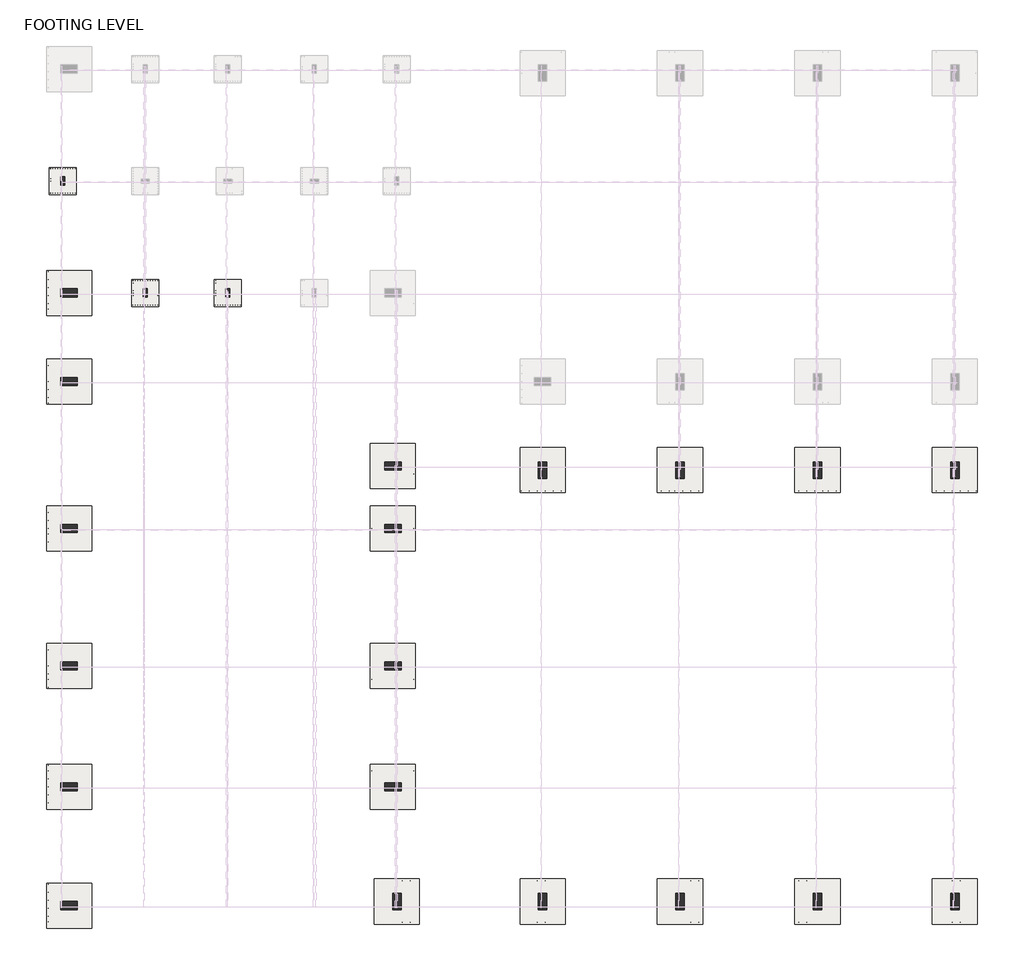
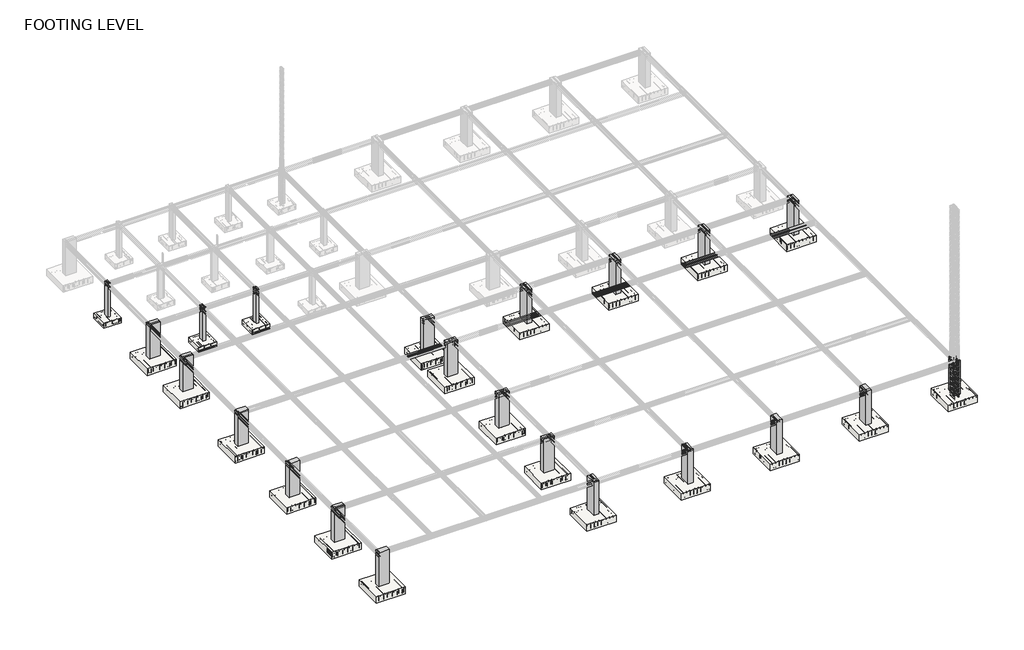
# One storey, part 1 of 19: 22 columns, 22 slabs.
"""IFC4 building model written with IfcOpenShell, lengths in millimetres."""

from ifc_helpers import new_model, si_unit, frame, origin, place, context, project, spatial, polyline, outline, extrude, faceted_brep, transform, mapped, element, save
from components import m_footing_rectangular_2500_x_2500_x_600_5d9c2050

model = new_model("IFC4")

# Units and contexts
model_context = context("Model", 3, world=origin())
ifc_project = project(units=[si_unit("LENGTHUNIT", "METRE", prefix="MILLI")], contexts=[model_context])

# Site, building, storey
site = spatial("IfcSite", under=ifc_project)
building = spatial("IfcBuilding", under=site)
storey = spatial("IfcBuildingStorey", under=building, Name="FOOTING LEVEL", Elevation=-3048.0)

# Columns
placement = place(None, origin())
element("IfcColumn", 1, ObjectType="M_Concrete-Rectangular-Column : 18\" X 36\"", at=placement, inside=storey, context=model_context, shape_type="SweptSolid", body=[
    extrude(outline(polyline([(32541.1587563, -27373.8205555), (32541.1587563, -28288.2205555), (32083.9587563, -28288.2205555), (32083.9587563, -27373.8205555), (32541.1587563, -27373.8205555)])), frame((0.0, 0.0, -3048.0), z_axis=(0.0, 0.0, 1.0), x_axis=(1.0, 0.0, 0.0)), (0.0, 0.0, 1.0), 3048.0),
])
element("IfcColumn", 2, ObjectType="M_Concrete-Rectangular-Column : 18\" X 36\"", at=placement, inside=storey, context=model_context, shape_type="SweptSolid", body=[
    extrude(outline(polyline([(24921.1587563, -27373.8205555), (24921.1587563, -28288.2205555), (24463.9587563, -28288.2205555), (24463.9587563, -27373.8205555), (24921.1587563, -27373.8205555)])), frame((0.0, 0.0, -3048.0), z_axis=(0.0, 0.0, 1.0), x_axis=(1.0, 0.0, 0.0)), (0.0, 0.0, 1.0), 3048.0),
])
element("IfcColumn", 3, ObjectType="M_Concrete-Rectangular-Column : 18\" X 36\"", at=placement, inside=storey, context=model_context, shape_type="Brep", body=[
    faceted_brep([(17301.1587563, -27373.8205555, -3048.0), (17301.1587563, -28288.2205555, -3048.0), (16843.9587563, -28288.2205555, -3048.0), (16843.9587563, -27373.8205555, -3048.0), (17301.1587563, -27373.8205555, 0.0), (17301.1587563, -27945.3205555, 0.0), (17301.1587563, -28173.9205555, 0.0), (17301.1587563, -28288.2205555, 0.0), (16843.9587563, -28288.2205555, 0.0), (16843.9587563, -28173.9205555, 0.0), (16843.9587563, -27945.3205555, 0.0), (16843.9587563, -27373.8205555, 0.0)], [[[0, 1, 2, 3]], [[4, 5, 6, 7, 1, 0]], [[7, 8, 2, 1]], [[8, 9, 10, 11, 3, 2]], [[11, 4, 0, 3]], [[4, 11, 10, 9, 8, 7, 6, 5]]]),
])
element("IfcColumn", 4, ObjectType="M_Concrete-Rectangular-Column : 18\" X 36\"", at=placement, inside=storey, context=model_context, shape_type="Brep", body=[
    faceted_brep([(9681.1587563, -27373.8205555, -3048.0), (9681.1587563, -28288.2205555, -3048.0), (9223.9587563, -28288.2205555, -3048.0), (9223.9587563, -27373.8205555, -3048.0), (9681.1587563, -27373.8205555, 0.0), (9681.1587563, -27945.3205555, 0.0), (9681.1587563, -28173.9205555, 0.0), (9681.1587563, -28288.2205555, 0.0), (9223.9587563, -28288.2205555, 0.0), (9223.9587563, -28173.9205555, 0.0), (9223.9587563, -27945.3205555, 0.0), (9223.9587563, -27373.8205555, 0.0)], [[[0, 1, 2, 3]], [[4, 5, 6, 7, 1, 0]], [[7, 8, 2, 1]], [[8, 9, 10, 11, 3, 2]], [[11, 4, 0, 3]], [[4, 11, 10, 9, 8, 7, 6, 5]]]),
])
element("IfcColumn", 5, ObjectType="M_Concrete-Rectangular-Column : 18\" X 36\"", at=placement, inside=storey, context=model_context, shape_type="SweptSolid", body=[
    extrude(outline(polyline([(1603.9587563, -27373.8205555), (1603.9587563, -28288.2205555), (1146.7587563, -28288.2205555), (1146.7587563, -27373.8205555), (1603.9587563, -27373.8205555)])), frame((0.0, 0.0, -3048.0), z_axis=(0.0, 0.0, 1.0), x_axis=(1.0, 0.0, 0.0)), (0.0, 0.0, 1.0), 3048.0),
])
element("IfcColumn", 6, ObjectType="M_Concrete-Rectangular-Column : 18\" X 36\"", at=placement, inside=storey, context=model_context, shape_type="SweptSolid", body=[
    extrude(outline(polyline([(-17255.5412437, -27831.0205555), (-16341.1412437, -27831.0205555), (-16341.1412437, -28288.2205555), (-17255.5412437, -28288.2205555), (-17255.5412437, -27831.0205555)])), frame((0.0, 0.0, -3048.0), z_axis=(0.0, 0.0, 1.0), x_axis=(1.0, 0.0, 0.0)), (0.0, 0.0, 1.0), 3048.0),
])
element("IfcColumn", 7, ObjectType="M_Concrete-Rectangular-Column : 18\" X 36\"", at=placement, inside=storey, context=model_context, shape_type="Brep", body=[
    faceted_brep([(-17255.5412437, -21239.7205555, -3048.0), (-16341.1412437, -21239.7205555, -3048.0), (-16341.1412437, -21696.9205555, -3048.0), (-17255.5412437, -21696.9205555, -3048.0), (-17255.5412437, -21239.7205555, 0.0), (-17026.9412437, -21239.7205555, 0.0), (-16341.1412437, -21239.7205555, 0.0), (-17255.5412437, -21239.7205555, -457.2), (-16341.1412437, -21696.9205555, 0.0), (-17026.9412437, -21696.9205555, 0.0), (-17255.5412437, -21696.9205555, 0.0), (-17255.5412437, -21696.9205555, -457.2)], [[[0, 1, 2, 3]], [[4, 5, 6, 1, 0, 7]], [[6, 8, 2, 1]], [[8, 9, 10, 11, 3, 2]], [[10, 4, 7, 0, 3, 11]], [[4, 10, 9, 8, 6, 5]]]),
])
element("IfcColumn", 8, ObjectType="M_Concrete-Rectangular-Column : 18\" X 36\"", at=placement, inside=storey, context=model_context, shape_type="Brep", body=[
    faceted_brep([(-17255.5412437, -14534.1205555, -3048.0), (-16341.1412437, -14534.1205555, -3048.0), (-16341.1412437, -14991.3205555, -3048.0), (-17255.5412437, -14991.3205555, -3048.0), (-17255.5412437, -14534.1205555, 0.0), (-17026.9412437, -14534.1205555, 0.0), (-16341.1412437, -14534.1205555, 0.0), (-17255.5412437, -14534.1205555, -457.2), (-16341.1412437, -14991.3205555, 0.0), (-17026.9412437, -14991.3205555, 0.0), (-17255.5412437, -14991.3205555, 0.0), (-17255.5412437, -14991.3205555, -457.2)], [[[0, 1, 2, 3]], [[4, 5, 6, 1, 0, 7]], [[6, 8, 2, 1]], [[8, 9, 10, 11, 3, 2]], [[10, 4, 7, 0, 3, 11]], [[4, 10, 9, 8, 6, 5]]]),
])
element("IfcColumn", 9, ObjectType="M_Concrete-Rectangular-Column : 18\" X 36\"", at=placement, inside=storey, context=model_context, shape_type="Brep", body=[
    faceted_brep([(-17255.5412437, -6914.1205555, -3048.0), (-16341.1412437, -6914.1205555, -3048.0), (-16341.1412437, -7371.3205555, -3048.0), (-17255.5412437, -7371.3205555, -3048.0), (-17255.5412437, -6914.1205555, 0.0), (-17026.9412437, -6914.1205555, 0.0), (-16341.1412437, -6914.1205555, 0.0), (-17255.5412437, -6914.1205555, -457.2), (-16341.1412437, -7371.3205555, 0.0), (-17026.9412437, -7371.3205555, 0.0), (-17255.5412437, -7371.3205555, 0.0), (-17255.5412437, -7371.3205555, -457.2)], [[[0, 1, 2, 3]], [[4, 5, 6, 1, 0, 7]], [[6, 8, 2, 1]], [[8, 9, 10, 11, 3, 2]], [[10, 4, 7, 0, 3, 11]], [[4, 10, 9, 8, 6, 5]]]),
])
element("IfcColumn", 10, ObjectType="M_Concrete-Rectangular-Column : 18\" X 36\"", at=placement, inside=storey, context=model_context, shape_type="Brep", body=[
    faceted_brep([(-17255.5412437, 1239.2794445, -3048.0), (-16341.1412437, 1239.2794445, -3048.0), (-16341.1412437, 782.0794445, -3048.0), (-17255.5412437, 782.0794445, -3048.0), (-17255.5412437, 1239.2794445, 0.0), (-17026.9412437, 1239.2794445, 0.0), (-16341.1412437, 1239.2794445, 0.0), (-17255.5412437, 1239.2794445, -457.2), (-16341.1412437, 782.0794445, 0.0), (-17026.9412437, 782.0794445, 0.0), (-17255.5412437, 782.0794445, 0.0), (-17255.5412437, 782.0794445, -457.2)], [[[0, 1, 2, 3]], [[4, 5, 6, 1, 0, 7]], [[6, 8, 2, 1]], [[8, 9, 10, 11, 3, 2]], [[10, 4, 7, 0, 3, 11]], [[4, 10, 9, 8, 6, 5]]]),
])
element("IfcColumn", 11, ObjectType="M_Concrete-Rectangular-Column : 18\" X 36\"", at=placement, inside=storey, context=model_context, shape_type="SweptSolid", body=[
    extrude(outline(polyline([(-17255.5412437, 6154.1794445), (-16341.1412437, 6154.1794445), (-16341.1412437, 5696.9794445), (-17255.5412437, 5696.9794445), (-17255.5412437, 6154.1794445)])), frame((0.0, 0.0, -3048.0), z_axis=(0.0, 0.0, 1.0), x_axis=(1.0, 0.0, 0.0)), (0.0, 0.0, 1.0), 3048.0),
])
element("IfcColumn", 12, ObjectType="M_Concrete-Rectangular-Column : 18\" X 36\"", at=placement, inside=storey, context=model_context, shape_type="Brep", body=[
    faceted_brep([(689.5587563, -3447.0205555, -3048.0), (1603.9587563, -3447.0205555, -3048.0), (1603.9587563, -3904.2205555, -3048.0), (689.5587563, -3904.2205555, -3048.0), (689.5587563, -3447.0205555, 0.0), (1261.0587563, -3447.0205555, 0.0), (1489.6587563, -3447.0205555, 0.0), (1603.9587563, -3447.0205555, 0.0), (1603.9587563, -3904.2205555, 0.0), (1489.6587563, -3904.2205555, 0.0), (1261.0587563, -3904.2205555, 0.0), (689.5587563, -3904.2205555, 0.0)], [[[0, 1, 2, 3]], [[4, 5, 6, 7, 1, 0]], [[7, 8, 2, 1]], [[8, 9, 10, 11, 3, 2]], [[11, 4, 0, 3]], [[4, 11, 10, 9, 8, 7, 6, 5]]]),
])
element("IfcColumn", 13, ObjectType="M_Concrete-Rectangular-Column : 18\" X 36\"", at=placement, inside=storey, context=model_context, shape_type="SweptSolid", body=[
    extrude(outline(polyline([(689.5587563, -6914.1205555), (1603.9587563, -6914.1205555), (1603.9587563, -7371.3205555), (689.5587563, -7371.3205555), (689.5587563, -6914.1205555)])), frame((0.0, 0.0, -3048.0), z_axis=(0.0, 0.0, 1.0), x_axis=(1.0, 0.0, 0.0)), (0.0, 0.0, 1.0), 3048.0),
])
element("IfcColumn", 14, ObjectType="M_Concrete-Rectangular-Column : 18\" X 36\"", at=placement, inside=storey, context=model_context, shape_type="Brep", body=[
    faceted_brep([(689.5587563, -14534.1205555, -3048.0), (1603.9587563, -14534.1205555, -3048.0), (1603.9587563, -14991.3205555, -3048.0), (689.5587563, -14991.3205555, -3048.0), (689.5587563, -14534.1205555, 0.0), (1261.0587563, -14534.1205555, 0.0), (1489.6587563, -14534.1205555, 0.0), (1603.9587563, -14534.1205555, 0.0), (1603.9587563, -14991.3205555, 0.0), (1489.6587563, -14991.3205555, 0.0), (1261.0587563, -14991.3205555, 0.0), (689.5587563, -14991.3205555, 0.0)], [[[0, 1, 2, 3]], [[4, 5, 6, 7, 1, 0]], [[7, 8, 2, 1]], [[8, 9, 10, 11, 3, 2]], [[11, 4, 0, 3]], [[4, 11, 10, 9, 8, 7, 6, 5]]]),
])
element("IfcColumn", 15, ObjectType="M_Concrete-Rectangular-Column : 18\" X 36\"", at=placement, inside=storey, context=model_context, shape_type="Brep", body=[
    faceted_brep([(689.5587563, -21239.7205555, -3048.0), (1603.9587563, -21239.7205555, -3048.0), (1603.9587563, -21696.9205555, -3048.0), (689.5587563, -21696.9205555, -3048.0), (689.5587563, -21239.7205555, 0.0), (1261.0587563, -21239.7205555, 0.0), (1489.6587563, -21239.7205555, 0.0), (1603.9587563, -21239.7205555, 0.0), (1603.9587563, -21696.9205555, 0.0), (1489.6587563, -21696.9205555, 0.0), (1261.0587563, -21696.9205555, 0.0), (689.5587563, -21696.9205555, 0.0)], [[[0, 1, 2, 3]], [[4, 5, 6, 7, 1, 0]], [[7, 8, 2, 1]], [[8, 9, 10, 11, 3, 2]], [[11, 4, 0, 3]], [[4, 11, 10, 9, 8, 7, 6, 5]]]),
])
element("IfcColumn", 16, ObjectType="M_Concrete-Rectangular-Column : 18\" X 36\"", at=placement, inside=storey, context=model_context, shape_type="Brep", body=[
    faceted_brep([(9223.9587563, -4361.4205555, -3048.0), (9223.9587563, -3447.0205555, -3048.0), (9681.1587563, -3447.0205555, -3048.0), (9681.1587563, -4361.4205555, -3048.0), (9223.9587563, -4361.4205555, 0.0), (9223.9587563, -3789.9205555, 0.0), (9223.9587563, -3561.3205555, 0.0), (9223.9587563, -3447.0205555, 0.0), (9681.1587563, -3447.0205555, 0.0), (9681.1587563, -3561.3205555, 0.0), (9681.1587563, -3789.9205555, 0.0), (9681.1587563, -4361.4205555, 0.0)], [[[0, 1, 2, 3]], [[4, 5, 6, 7, 1, 0]], [[7, 8, 2, 1]], [[8, 9, 10, 11, 3, 2]], [[11, 4, 0, 3]], [[4, 11, 10, 9, 8, 7, 6, 5]]]),
])
element("IfcColumn", 17, ObjectType="M_Concrete-Rectangular-Column : 18\" X 36\"", at=placement, inside=storey, context=model_context, shape_type="Brep", body=[
    faceted_brep([(16843.9587563, -4361.4205555, -3048.0), (16843.9587563, -3447.0205555, -3048.0), (17301.1587563, -3447.0205555, -3048.0), (17301.1587563, -4361.4205555, -3048.0), (16843.9587563, -4361.4205555, 0.0), (16843.9587563, -3789.9205555, 0.0), (16843.9587563, -3561.3205555, 0.0), (16843.9587563, -3447.0205555, 0.0), (17301.1587563, -3447.0205555, 0.0), (17301.1587563, -3561.3205555, 0.0), (17301.1587563, -3789.9205555, 0.0), (17301.1587563, -4361.4205555, 0.0)], [[[0, 1, 2, 3]], [[4, 5, 6, 7, 1, 0]], [[7, 8, 2, 1]], [[8, 9, 10, 11, 3, 2]], [[11, 4, 0, 3]], [[4, 11, 10, 9, 8, 7, 6, 5]]]),
])
element("IfcColumn", 18, ObjectType="M_Concrete-Rectangular-Column : 18\" X 36\"", at=placement, inside=storey, context=model_context, shape_type="SweptSolid", body=[
    extrude(outline(polyline([(24463.9587563, -4361.4205555), (24463.9587563, -3447.0205555), (24921.1587563, -3447.0205555), (24921.1587563, -4361.4205555), (24463.9587563, -4361.4205555)])), frame((0.0, 0.0, -3048.0), z_axis=(0.0, 0.0, 1.0), x_axis=(1.0, 0.0, 0.0)), (0.0, 0.0, 1.0), 3048.0),
])
element("IfcColumn", 19, ObjectType="M_Concrete-Rectangular-Column : 18\" X 36\"", at=placement, inside=storey, context=model_context, shape_type="SweptSolid", body=[
    extrude(outline(polyline([(32083.9587563, -4361.4205555), (32083.9587563, -3447.0205555), (32541.1587563, -3447.0205555), (32541.1587563, -4361.4205555), (32083.9587563, -4361.4205555)])), frame((0.0, 0.0, -3048.0), z_axis=(0.0, 0.0, 1.0), x_axis=(1.0, 0.0, 0.0)), (0.0, 0.0, 1.0), 3048.0),
])
element("IfcColumn", 20, ObjectType="M_Concrete-Rectangular-Column : 9\" X18\"", at=placement, inside=storey, context=model_context, shape_type="Brep", body=[
    faceted_brep([(-12683.5412437, 5696.9794445, -3048.0), (-12683.5412437, 6154.1794445, -3048.0), (-12454.9412437, 6154.1794445, -3048.0), (-12454.9412437, 5696.9794445, -3048.0), (-12683.5412437, 5696.9794445, 0.0), (-12683.5412437, 5811.2794445, 0.0), (-12683.5412437, 6039.8794445, 0.0), (-12683.5412437, 6154.1794445, 0.0), (-12683.5412437, 6154.1794445, -457.2), (-12454.9412437, 6154.1794445, 0.0), (-12454.9412437, 6154.1794445, -457.2), (-12454.9412437, 6039.8794445, 0.0), (-12454.9412437, 5811.2794445, 0.0), (-12454.9412437, 5696.9794445, 0.0)], [[[0, 1, 2, 3]], [[4, 5, 6, 7, 8, 1, 0]], [[7, 9, 10, 2, 1, 8]], [[9, 11, 12, 13, 3, 2, 10]], [[13, 4, 0, 3]], [[4, 13, 12, 11, 9, 7, 6, 5]]]),
])
element("IfcColumn", 21, ObjectType="M_Concrete-Rectangular-Column : 9\" X18\"", at=placement, inside=storey, context=model_context, shape_type="Brep", body=[
    faceted_brep([(-8111.5412437, 5696.9794445, -3048.0), (-8111.5412437, 6154.1794445, -3048.0), (-7882.9412437, 6154.1794445, -3048.0), (-7882.9412437, 5696.9794445, -3048.0), (-8111.5412437, 5696.9794445, 0.0), (-8111.5412437, 5811.2794445, 0.0), (-8111.5412437, 6039.8794445, 0.0), (-8111.5412437, 6154.1794445, 0.0), (-8111.5412437, 6154.1794445, -457.2), (-7882.9412437, 6154.1794445, 0.0), (-7882.9412437, 6154.1794445, -457.2), (-7882.9412437, 6039.8794445, 0.0), (-7882.9412437, 5811.2794445, 0.0), (-7882.9412437, 5696.9794445, 0.0)], [[[0, 1, 2, 3]], [[4, 5, 6, 7, 8, 1, 0]], [[7, 9, 10, 2, 1, 8]], [[9, 11, 12, 13, 3, 2, 10]], [[13, 4, 0, 3]], [[4, 13, 12, 11, 9, 7, 6, 5]]]),
])
element("IfcColumn", 22, ObjectType="M_Concrete-Rectangular-Column : 9\" X18\"", at=placement, inside=storey, context=model_context, shape_type="Brep", body=[
    faceted_brep([(-17255.5412437, 11907.2794445, -3048.0), (-17255.5412437, 12364.4794445, -3048.0), (-17026.9412437, 12364.4794445, -3048.0), (-17026.9412437, 11907.2794445, -3048.0), (-17255.5412437, 11907.2794445, 0.0), (-17255.5412437, 12364.4794445, 0.0), (-17255.5412437, 12364.4794445, -457.2), (-17255.5412437, 11907.2794445, -457.2), (-17026.9412437, 12364.4794445, 0.0), (-17026.9412437, 12364.4794445, -457.2), (-17026.9412437, 11907.2794445, 0.0), (-17026.9412437, 11907.2794445, -457.2)], [[[0, 1, 2, 3]], [[4, 5, 6, 1, 0, 7]], [[5, 8, 9, 2, 1, 6]], [[8, 10, 11, 3, 2, 9]], [[10, 4, 7, 0, 3, 11]], [[4, 10, 8, 5]]]),
])

# Slabs
element("IfcSlab", 23, ObjectType="M_Footing-Rectangular : 1500 X1500 X450", at=placement, inside=storey, context=model_context, shape_type="SweptSolid", body=[
    extrude(outline(polyline([(-11819.2412437, 6675.5794445), (-11819.2412437, 5175.5794445), (-13319.2412437, 5175.5794445), (-13319.2412437, 6675.5794445), (-11819.2412437, 6675.5794445)])), frame((0.0, 0.0, -3498.0), z_axis=(0.0, 0.0, 1.0), x_axis=(1.0, 0.0, 0.0)), (0.0, 0.0, 1.0), 450.0),
])
element("IfcSlab", 24, ObjectType="M_Footing-Rectangular : 1500 X1500 X450", at=placement, inside=storey, context=model_context, shape_type="SweptSolid", body=[
    extrude(outline(polyline([(-7247.2412437, 6675.5794445), (-7247.2412437, 5175.5794445), (-8747.2412437, 5175.5794445), (-8747.2412437, 6675.5794445), (-7247.2412437, 6675.5794445)])), frame((0.0, 0.0, -3498.0), z_axis=(0.0, 0.0, 1.0), x_axis=(1.0, 0.0, 0.0)), (0.0, 0.0, 1.0), 450.0),
])
element("IfcSlab", 25, ObjectType="M_Footing-Rectangular : 1500 X1500 X450", at=placement, inside=storey, context=model_context, shape_type="SweptSolid", body=[
    extrude(outline(polyline([(-16391.2412437, 12885.8794445), (-16391.2412437, 11385.8794445), (-17891.2412437, 11385.8794445), (-17891.2412437, 12885.8794445), (-16391.2412437, 12885.8794445)])), frame((0.0, 0.0, -3498.0), z_axis=(0.0, 0.0, 1.0), x_axis=(1.0, 0.0, 0.0)), (0.0, 0.0, 1.0), 450.0),
])
element("IfcSlab", 26, ObjectType="M_Footing-Rectangular : 2500 X 2500 X 600", at=placement, inside=storey, context=model_context, shape_type="SweptSolid", body=[
    extrude(outline(polyline([(-15548.3412437, 7175.5794445), (-15548.3412437, 4675.5794445), (-18048.3412437, 4675.5794445), (-18048.3412437, 7175.5794445), (-15548.3412437, 7175.5794445)])), frame((0.0, 0.0, -3648.0), z_axis=(0.0, 0.0, 1.0), x_axis=(1.0, 0.0, 0.0)), (0.0, 0.0, 1.0), 600.0),
])
m_footing_rectangular_2500_x_2500_x_600_shape = m_footing_rectangular_2500_x_2500_x_600_5d9c2050(model_context)
element("IfcSlab", 27, ObjectType="M_Footing-Rectangular : 2500 X 2500 X 600", at=placement, inside=storey, context=model_context, shape_type="MappedRepresentation", body=[
    mapped(m_footing_rectangular_2500_x_2500_x_600_shape, transform((-16798.3412437, -28059.6205555, -3048.0), x_axis=(1.0, 0.0, 0.0), y_axis=(0.0, 1.0, 0.0), z_axis=(0.0, 0.0, 1.0))),
])
element("IfcSlab", 28, ObjectType="M_Footing-Rectangular : 2500 X 2500 X 600", at=placement, inside=storey, context=model_context, shape_type="MappedRepresentation", body=[
    mapped(m_footing_rectangular_2500_x_2500_x_600_shape, transform((1375.3587563, -27831.0205555, -3048.0), x_axis=(1.0, 0.0, 0.0), y_axis=(0.0, 1.0, 0.0), z_axis=(0.0, 0.0, 1.0))),
])
element("IfcSlab", 29, ObjectType="M_Footing-Rectangular : 2500 X 2500 X 600", at=placement, inside=storey, context=model_context, shape_type="MappedRepresentation", body=[
    mapped(m_footing_rectangular_2500_x_2500_x_600_shape, transform((9452.5587563, -27831.0205555, -3048.0), x_axis=(1.0, 0.0, 0.0), y_axis=(0.0, 1.0, 0.0), z_axis=(0.0, 0.0, 1.0))),
])
element("IfcSlab", 30, ObjectType="M_Footing-Rectangular : 2500 X 2500 X 600", at=placement, inside=storey, context=model_context, shape_type="MappedRepresentation", body=[
    mapped(m_footing_rectangular_2500_x_2500_x_600_shape, transform((17072.5587563, -27831.0205555, -3048.0), x_axis=(1.0, 0.0, 0.0), y_axis=(0.0, 1.0, 0.0), z_axis=(0.0, 0.0, 1.0))),
])
element("IfcSlab", 31, ObjectType="M_Footing-Rectangular : 2500 X 2500 X 600", at=placement, inside=storey, context=model_context, shape_type="MappedRepresentation", body=[
    mapped(m_footing_rectangular_2500_x_2500_x_600_shape, transform((24692.5587563, -27831.0205555, -3048.0), x_axis=(1.0, 0.0, 0.0), y_axis=(0.0, 1.0, 0.0), z_axis=(0.0, 0.0, 1.0))),
])
element("IfcSlab", 32, ObjectType="M_Footing-Rectangular : 2500 X 2500 X 600", at=placement, inside=storey, context=model_context, shape_type="MappedRepresentation", body=[
    mapped(m_footing_rectangular_2500_x_2500_x_600_shape, transform((32312.5587563, -27831.0205555, -3048.0), x_axis=(1.0, 0.0, 0.0), y_axis=(0.0, 1.0, 0.0), z_axis=(0.0, 0.0, 1.0))),
])
element("IfcSlab", 33, ObjectType="M_Footing-Rectangular : 2500 X 2500 X 600", at=placement, inside=storey, context=model_context, shape_type="MappedRepresentation", body=[
    mapped(m_footing_rectangular_2500_x_2500_x_600_shape, transform((-16798.3412437, -21468.3205555, -3048.0), x_axis=(1.0, 0.0, 0.0), y_axis=(0.0, 1.0, 0.0), z_axis=(0.0, 0.0, 1.0))),
])
element("IfcSlab", 34, ObjectType="M_Footing-Rectangular : 2500 X 2500 X 600", at=placement, inside=storey, context=model_context, shape_type="MappedRepresentation", body=[
    mapped(m_footing_rectangular_2500_x_2500_x_600_shape, transform((1146.7587563, -21468.3205555, -3048.0), x_axis=(1.0, 0.0, 0.0), y_axis=(0.0, 1.0, 0.0), z_axis=(0.0, 0.0, 1.0))),
])
element("IfcSlab", 35, ObjectType="M_Footing-Rectangular : 2500 X 2500 X 600", at=placement, inside=storey, context=model_context, shape_type="MappedRepresentation", body=[
    mapped(m_footing_rectangular_2500_x_2500_x_600_shape, transform((1146.7587563, -14762.7205555, -3048.0), x_axis=(1.0, 0.0, 0.0), y_axis=(0.0, 1.0, 0.0), z_axis=(0.0, 0.0, 1.0))),
])
element("IfcSlab", 36, ObjectType="M_Footing-Rectangular : 2500 X 2500 X 600", at=placement, inside=storey, context=model_context, shape_type="MappedRepresentation", body=[
    mapped(m_footing_rectangular_2500_x_2500_x_600_shape, transform((-16798.3412437, -14762.7205555, -3048.0), x_axis=(1.0, 0.0, 0.0), y_axis=(0.0, 1.0, 0.0), z_axis=(0.0, 0.0, 1.0))),
])
element("IfcSlab", 37, ObjectType="M_Footing-Rectangular : 2500 X 2500 X 600", at=placement, inside=storey, context=model_context, shape_type="MappedRepresentation", body=[
    mapped(m_footing_rectangular_2500_x_2500_x_600_shape, transform((-16798.3412437, -7142.7205555, -3048.0), x_axis=(1.0, 0.0, 0.0), y_axis=(0.0, 1.0, 0.0), z_axis=(0.0, 0.0, 1.0))),
])
element("IfcSlab", 38, ObjectType="M_Footing-Rectangular : 2500 X 2500 X 600", at=placement, inside=storey, context=model_context, shape_type="MappedRepresentation", body=[
    mapped(m_footing_rectangular_2500_x_2500_x_600_shape, transform((-16798.3412437, 1010.6794445, -3048.0), x_axis=(1.0, 0.0, 0.0), y_axis=(0.0, 1.0, 0.0), z_axis=(0.0, 0.0, 1.0))),
])
element("IfcSlab", 39, ObjectType="M_Footing-Rectangular : 2500 X 2500 X 600", at=placement, inside=storey, context=model_context, shape_type="MappedRepresentation", body=[
    mapped(m_footing_rectangular_2500_x_2500_x_600_shape, transform((1146.7587563, -3675.6205555, -3048.0), x_axis=(1.0, 0.0, 0.0), y_axis=(0.0, 1.0, 0.0), z_axis=(0.0, 0.0, 1.0))),
])
element("IfcSlab", 40, ObjectType="M_Footing-Rectangular : 2500 X 2500 X 600", at=placement, inside=storey, context=model_context, shape_type="MappedRepresentation", body=[
    mapped(m_footing_rectangular_2500_x_2500_x_600_shape, transform((1146.7587563, -7142.7205555, -3048.0), x_axis=(1.0, 0.0, 0.0), y_axis=(0.0, 1.0, 0.0), z_axis=(0.0, 0.0, 1.0))),
])
element("IfcSlab", 41, ObjectType="M_Footing-Rectangular : 2500 X 2500 X 600", at=placement, inside=storey, context=model_context, shape_type="MappedRepresentation", body=[
    mapped(m_footing_rectangular_2500_x_2500_x_600_shape, transform((9452.5587563, -3904.2205555, -3048.0), x_axis=(1.0, 0.0, 0.0), y_axis=(0.0, 1.0, 0.0), z_axis=(0.0, 0.0, 1.0))),
])
element("IfcSlab", 42, ObjectType="M_Footing-Rectangular : 2500 X 2500 X 600", at=placement, inside=storey, context=model_context, shape_type="MappedRepresentation", body=[
    mapped(m_footing_rectangular_2500_x_2500_x_600_shape, transform((17072.5587563, -3904.2205555, -3048.0), x_axis=(1.0, 0.0, 0.0), y_axis=(0.0, 1.0, 0.0), z_axis=(0.0, 0.0, 1.0))),
])
element("IfcSlab", 43, ObjectType="M_Footing-Rectangular : 2500 X 2500 X 600", at=placement, inside=storey, context=model_context, shape_type="MappedRepresentation", body=[
    mapped(m_footing_rectangular_2500_x_2500_x_600_shape, transform((24692.5587563, -3904.2205555, -3048.0), x_axis=(1.0, 0.0, 0.0), y_axis=(0.0, 1.0, 0.0), z_axis=(0.0, 0.0, 1.0))),
])
element("IfcSlab", 44, ObjectType="M_Footing-Rectangular : 2500 X 2500 X 600", at=placement, inside=storey, context=model_context, shape_type="MappedRepresentation", body=[
    mapped(m_footing_rectangular_2500_x_2500_x_600_shape, transform((32312.5587563, -3904.2205555, -3048.0), x_axis=(1.0, 0.0, 0.0), y_axis=(0.0, 1.0, 0.0), z_axis=(0.0, 0.0, 1.0))),
])

save(model, "model.ifc")

# Revit data of these elements
# Grids (mm)
#   "A": line (-17141.241, -35283.407) -> (-17141.241, 24480.414)
#   "1": line (40763.342, -28059.621) -> (-25632.078, -28059.621)
#   "3": line (40763.342, 18346.179) -> (-25632.078, 18346.179)
#   "B": line (1375.359, -35283.407) -> (1375.359, 24480.414)
#   "C": line (9452.559, 24480.414) -> (9452.559, -35283.407)
#   "D": line (17072.559, 24480.414) -> (17072.559, -35283.407)
#   "E": line (24692.559, 24480.414) -> (24692.559, -35283.407)
#   "F": line (32312.559, 24480.414) -> (32312.559, -35283.407)
#   "a": line (6286.814, -21468.321) -> (-25632.078, -21468.321)
#   "b": line (6286.814, -14762.721) -> (-25632.078, -14762.721)
#   "c": line (6286.814, -7142.721) -> (-25632.078, -7142.721)
#   "2": line (40763.342, 1010.679) -> (-25632.078, 1010.679)
#   "X": line (6286.814, 5925.579) -> (-25632.078, 5925.579)
#   "Y": line (6286.814, 12135.879) -> (-25632.078, 12135.879)
#   "G": line (40763.342, -3675.621) -> (-3184.634, -3675.621)
#   "XX": line (-12569.241, 24480.414) -> (-12569.241, 4225.579)
#   "YY": line (-7997.241, 4225.579) -> (-7997.241, 24480.414)
#   "ZZ": line (-3196.641, 4225.579) -> (-3196.641, 24480.414)
# Type "M_Concrete-Rectangular-Column : 18\" X 36\""
#   b = 457.2 mm
#   h = 914.4 mm
#   Structural Material [instance default] = Concrete, Cast-in-Place gray
# Type "M_Concrete-Rectangular-Column : 9\" X18\""
#   b = 228.6 mm
#   h = 457.2 mm
#   Structural Material [instance default] = Concrete, Cast-in-Place gray
# Type "M_Footing-Rectangular : 1500 X1500 X450"
#   Width = 1500 mm
#   Length = 1500 mm
#   Foundation Thickness = 450 mm
#   Structural Material [instance default] = Concrete, Cast-in-Place gray
#   Assembly Code = ""
# Type "M_Footing-Rectangular : 2500 X 2500 X 600"
#   Width = 2500 mm
#   Length = 2500 mm
#   Foundation Thickness = 600 mm
#   Structural Material [instance default] = Concrete, Cast-in-Place gray
#   Assembly Code = ""
# Elements 1, 2, 3, 4, 5, 6, 7, 8, 9, 10, 11, 12, 13, 14, 15, 16, 17, 18, 19 (IfcColumn, "M_Concrete-Rectangular-Column : 18\" X 36\"")
#   Structural Material = Concrete, Cast-in-Place gray
#   Phase Created = New Construction
#   Materials on its faces: "Concrete, Cast-in-Place gray"
# Elements 20, 21, 22 (IfcColumn, "M_Concrete-Rectangular-Column : 9\" X18\"")
#   Structural Material = Concrete, Cast-in-Place gray
#   Phase Created = New Construction
#   Materials on its faces: "Concrete, Cast-in-Place gray"
# Elements 23, 24, 25 (IfcSlab, "M_Footing-Rectangular : 1500 X1500 X450")
#   Structural Material = Concrete, Cast-in-Place gray
#   Phase Created = New Construction
#   Materials on its faces: "Concrete, Cast-in-Place gray"
# Elements 26, 27, 28, 29, 30, 31, 32, 33, 34, 35, 36, 37, 38, 39, 40, 41, 42, 43, 44 (IfcSlab, "M_Footing-Rectangular : 2500 X 2500 X 600")
#   Structural Material = Concrete, Cast-in-Place gray
#   Phase Created = New Construction
#   Materials on its faces: "Concrete, Cast-in-Place gray"
# Materials
#   "Concrete, Cast-in-Place gray": class "Concrete", colour RGB 192 192 192, transparency 0, Description = "Cast-in-place concrete", Cost = 0
